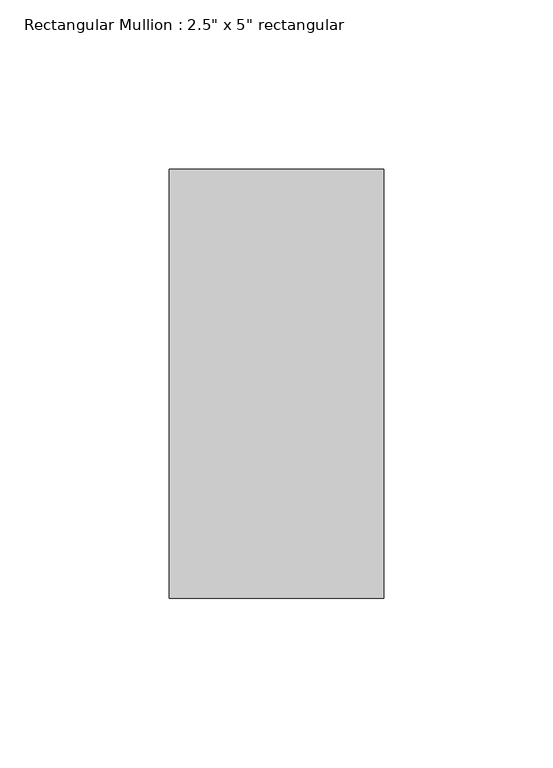
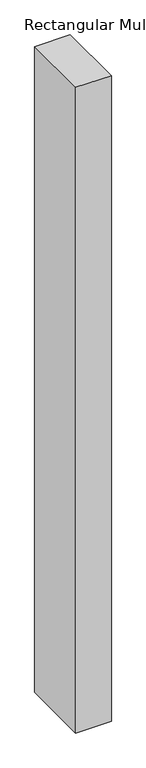
"""IFC4 building model written with IfcOpenShell, lengths in millimetres: member geometry."""

from ifc_helpers import new_model, si_unit, frame, origin, place, context, project, spatial, polyline, outline, extrude, source, transform, mapped, element, save


def member_667b8694(model_context):
    return source(origin(), model_context, "Body", "SweptSolid", [
        extrude(outline(polyline([(31.75, 63.5), (31.75, -63.5), (-31.75, -63.5), (-31.75, 63.5), (31.75, 63.5)])), frame((0.0, 0.0, -1219.1999999), z_axis=(0.0, 0.0, 1.0), x_axis=(1.0, 0.0, 0.0)), (0.0, 0.0, 1.0), 1219.1999999),
    ])


if __name__ == "__main__":
    model = new_model("IFC4")
    model_context = context("Model", 3, world=origin())
    ifc_project = project(units=[si_unit("LENGTHUNIT", "METRE", prefix="MILLI")], contexts=[model_context])
    site = spatial("IfcSite", under=ifc_project)
    building = spatial("IfcBuilding", under=site)
    placement = place(None, origin())
    member_shape = member_667b8694(model_context)
    element("IfcMember", 1, ObjectType="Rectangular Mullion : 2.5\" x 5\" rectangular", at=placement, inside=building, context=model_context, shape_type="MappedRepresentation", body=[
        mapped(member_shape, transform((0.0, 0.0, 0.0), x_axis=(1.0, 0.0, 0.0), y_axis=(0.0, 1.0, 0.0), z_axis=(0.0, 0.0, 1.0))),
    ])
    save(model, "model.ifc")

# Revit data of these elements
# Type "Rectangular Mullion : 2.5\" x 5\" rectangular"
#   built-in parameter 1007304 = 0.416667 (stored number, unit not read)
#   built-in parameter 1007301 = 0.104167 (stored number, unit not read)
#   built-in parameter 1007300 = 0.104167 (stored number, unit not read)
# Element 1 (IfcMember, "Rectangular Mullion : 2.5\" x 5\" rectangular")
#   Materials on its faces: "Aluminum"
# Materials
#   "Aluminum": class "Metal", colour RGB 247 247 247, transparency 0, Description = "Aluminum 6061", Cost = 0
